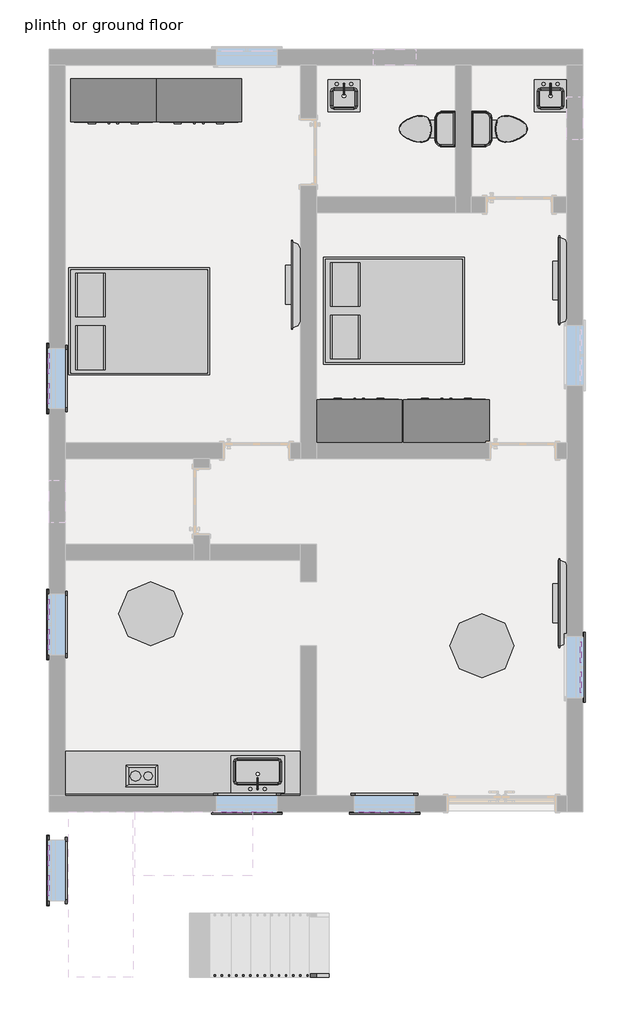
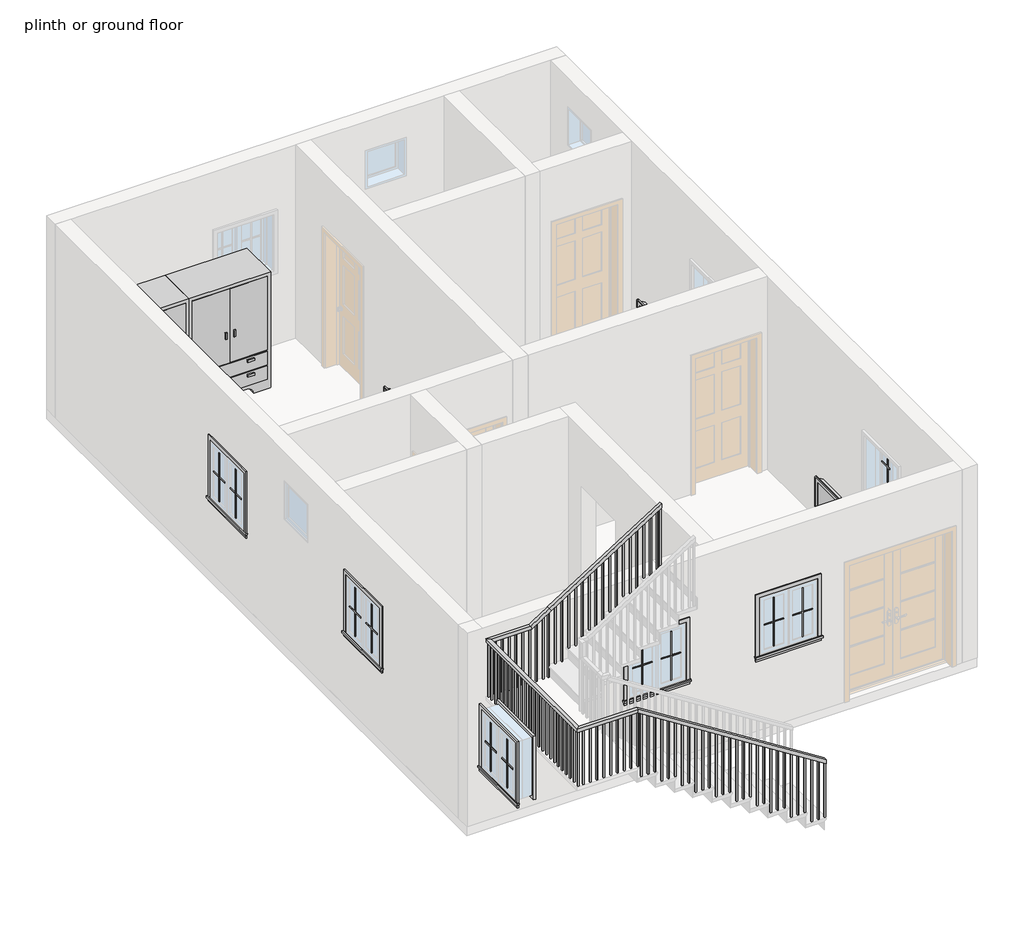
# One storey, part 2 of 3: 24 proxies, 12 furniture elements, 5 flow terminals, 1 railing.
# Revit data of these elements (continued)
# Element 37 (IfcFurniture, "Table-Dining Round w Chairs : 36\" Diameter") (continued)
#   Materials on its faces: "Pine", "Laminate, Linen, Matte"
# Elements 38, 39, 40, 41 (IfcFurniture, "Wardrobe : 48\" x 72\" x 24\"")
#   Phase Created = New Construction
#   Materials on its faces: "Wood - Mahogany"
# Element 42 (IfcRailing, "Handrail - Rectangular")
#   Phase Created = New Construction
# Materials
#   "Metal - Chrome": colour RGB 17 17 17, transparency 0
#   "Metal - Steel, Polished": colour RGB 57 57 57, transparency 0
#   "Steel, Polished": class "Metal", colour RGB 57 57 57, transparency 0, Description = "Polished steel", Cost = 0
#   "Porcelain, Linen": class "Ceramic", colour RGB 249 239 230, transparency 0, Description = "Porcelain, linen", Cost = 0
#   "Laminate, Linen, Matte": class "Plastic", colour RGB 249 239 230, transparency 0, Description = "Plastic Laminate - Linen, Matte", Cost = 0
#   "Birch": class "Wood", colour RGB 224 178 126, transparency 0, Description = "Betula Alleghaniensis", Cost = 0
#   "Linen, White": class "Textile", colour RGB 247 247 239, transparency 0, Description = "Linen, white", Cost = 0
#   "Pine": class "Wood", colour RGB 223 192 134, transparency 0, Description = "Pinus Echinata", Cost = 0
#   "Wood - Mahogany": colour RGB 138 86 45, transparency 0
#   "Clad - White": class "Wood", colour RGB 242 242 238, transparency 0, Cost = 0
#   "Wood - Stained": class "Wood", colour RGB 224 178 126, transparency 0, Cost = 0
#   "Counter Top": class "Wood", colour RGB 226 177 128, transparency 0
#   "TV - Black": colour RGB 49 49 49, transparency 0
#   "TV - Glass": colour RGB 157 157 157, transparency 0.9
#   "TV - Screen": colour RGB 0 0 0, transparency 0
